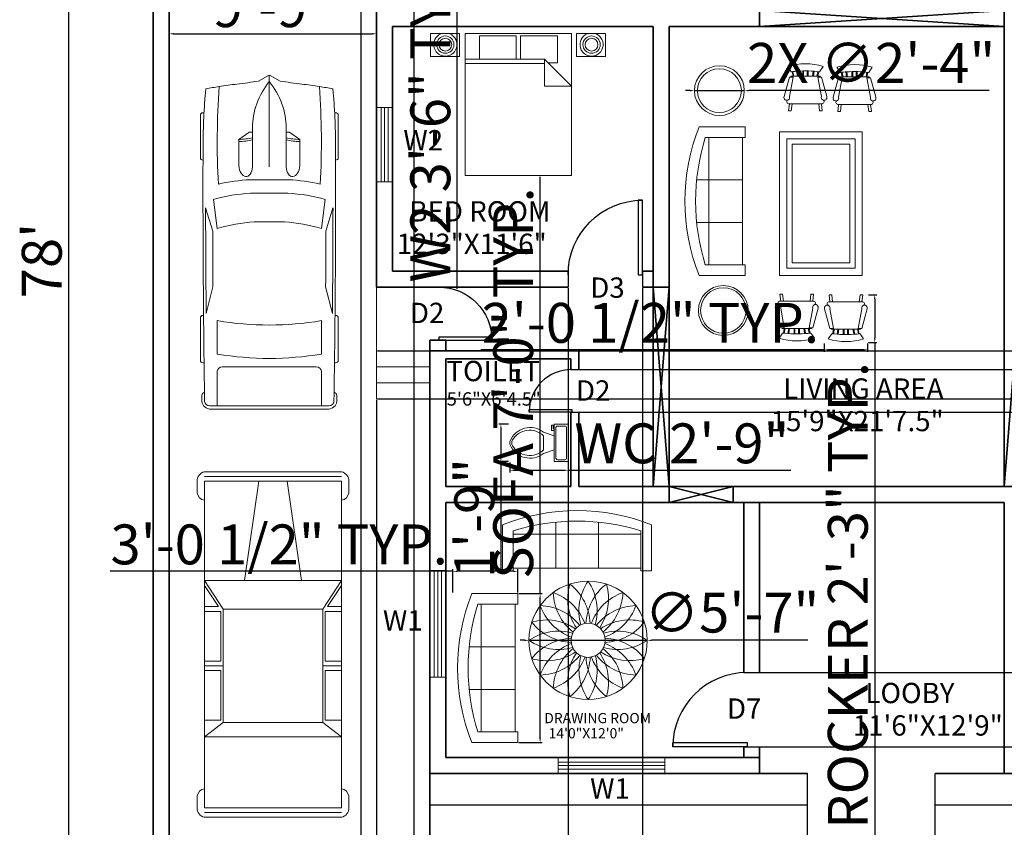
# Model space of a CAD drawing. Units: inches. Extents: x 164 to 1038, y 98 to 1358.
# Tile 2 of 4: x 199 to 754, y 358 to 814. Entities that reach past the tile are written whole.
import ezdxf

# ---------------------------------------------------------------- set-up
doc = ezdxf.new("R2010")
doc.units = ezdxf.units.IN
for name, color, linetype, lineweight in [('A-ANNO-DIMS', 7, 'Continuous', 18), ('A-ANNO-TEXT', 3, 'Continuous', 18), ('A-AREA-IDEN', 3, 'Continuous', 18), ('A-FLOR', 7, 'Continuous', 25), ('A-FLOR-FIXT', 2, 'Continuous', 18), ('C-SITE-VEHI', 2, 'Continuous', 13), ('C-SITE-WALL', 7, 'Continuous', 35), ('door', 6, 'Continuous', 25), ('furniture', 2, 'Continuous', 18), ('staircase', 4, 'Continuous', 18), ('wall', 7, 'Continuous', 35), ('window', 10, 'Continuous', 18)]:
    doc.layers.add(name, color=color, linetype=linetype, lineweight=lineweight)
doc.styles.get("Standard").update_dxf_attribs({"font": 'arial.ttf'})
doc.dimstyles.new('ISO-25', dxfattribs={"dimtxt": 22.5, "dimasz": 2.5, "dimexe": 1.25, "dimexo": 0.625, "dimtad": 1, "dimdec": 0, "dimlunit": 3, "dimtxsty": 'Standard', "dimcen": 2.5, "dimadec": 0, "dimazin": 0, "dimtfac": 1, "dimtdec": 0, "dimtmove": 0, "dimatfit": 3, "dimfxl": 1, "dimarcsym": 0})

# ---------------------------------------------------------------- blocks, each defined once
blk = doc.blocks.new('*U3')
for p, q in [((0, 0), (0, -5)), ((30, 0), (30, -5))]:
    blk.add_line(p, q)
blk.add_lwpolyline([(0, 0), (0, 30), (1.75, 30), (1.75, 0)], close=True)
blk.add_arc((0, 0), 30, 0, 90)
blk = doc.blocks.new('Bed - Queen')
for p, q in [((0, -80.00003), (0, 0)), ((0, 0), (59.99999, 0)), ((59.99999, 0), (59.99999, -80.00003)), ((7.99999, -1.2), (28.79998, -1.2)), ((7.99999, -14.4), (7.99999, -1.2)), ((28.79998, -1.2), (28.79998, -14.4)), ((31.19999, -1.2), (51.99999, -1.2)), ((31.19999, -14.4), (31.19999, -1.2)), ((51.99999, -1.2), (51.99999, -16.4)), ((0, -14.4), (44.8, -14.4)), ((59.99999, -29.6), (44.8, -14.4)), ((44.8, -14.4), (44.8, -29.6)), ((51.99999, -16.4), (46.79936, -16.4)), ((44.8, -16.8), (0, -16.8)), ((44.8, -29.6), (59.99999, -29.6)), ((59.99999, -80.00003), (0, -80.00003))]:
    blk.add_line(p, q)
blk = doc.blocks.new('Toilet - top')
for p, q in [((9.5, -6), (9.5, -2)), ((-10, -8.5), (-8, -8.5)), ((-10, -9.5), (-10, -8.5)), ((-7, -9.5), (-10, -9.5)), ((-8, -8.5), (-8, -8)), ((-7, -8), (-7, -9.5)), ((-4, -8), (-6, -14)), ((4, -8), (6, -14)), ((4, -14), (-4, -14))]:
    blk.add_line(p, q)
blk.add_lwpolyline([(10.5, -8), (10.5, 0), (-10.5, 0), (-10.5, -8)], close=True)
for points in [[(-9.5, -2), (-9.5, -6)], [(8.5, -1), (-8.5, -1)], [(-8.5, -7), (8.5, -7)]]:
    blk.add_lwpolyline(points)
for centre, radius, start, end in [((-8.62, -1.88), 0.884, 81.8699, 188.1301), ((8.62, -1.88), 0.884, 351.8699, 98.1301), ((-8.62, -6.12), 0.884, 171.8699, 278.1301), ((8.62, -6.12), 0.884, 261.8699, 8.1301), ((3.52, -21.58), 12.17, 141.4691, 247.9714), ((4.2, -21.82), 11.33, 136.3677, 238.9468), ((-3.52, -21.58), 12.17, 292.0284, 38.5307), ((-4.2, -21.82), 11.33, 301.053, 43.6321), ((0, -27.88), 4, 245.7318, 294.2682), ((0, -29), 4, 254.8605, 285.1395)]:
    blk.add_arc(centre, radius, start, end)
blk = doc.blocks.new('Sofa - Roundback 7 ft.')
for p, q in [((-12.00002, -32.4421), (-12.00003, -6.5971)), ((11.99997, -32.4421), (11.99998, -6.5971)), ((-36.000027, -34), (-36.000027, -11.4696)), ((-35.999844, -13.3819), (35.9998, -13.3819)), ((35.99998, -34), (35.99998, -11.4696)), ((-36.000027, -32.4421), (35.99998, -32.4421))]:
    blk.add_line(p, q)
for points in [[(-36.000027, -34), (-42.000027, -34), (-42.000027, -8)], [(41.99998, -8), (41.99998, -34), (35.99998, -34)]]:
    blk.add_lwpolyline(points)
for centre, radius, start, end in [((0, -114.25), 114.25, 68.43141, 111.5686), ((-0.00001, -127.1968), 121.1968, 72.72033, 107.2797)]:
    blk.add_arc(centre, radius, start, end)
blk = doc.blocks.new('Chair - Rocking')
for p, q in [((-8, -4.5), (-10, -1.5)), ((-7.5, -4.5), (-7, -7)), ((-6.5, -7), (-7.02225, -4.43)), ((-4.5, -7), (-4.96674, -4.19951)), ((-4, -7), (-4.40532, -4.16272)), ((-1.5, -4.05012), (-1.5, -7)), ((-1, -7), (-1, -4.05012)), ((1, -7), (1, -4.04655)), ((1.5, -4.05012), (1.5, -7)), ((4, -7), (4.40187, -4.18694)), ((4.5, -7), (4.96761, -4.19437)), ((6.5, -7), (7, -4.4057)), ((7.5, -4.5), (7, -7)), ((8, -4.5), (10, -1.5)), ((-9, -7.5), (-12, -18.49999)), ((-7, -7.5), (-9, -7.5)), ((-9, -18.49999), (-7, -7.5)), ((-8.23428, -6.99939), (-8.3093, -7.47958)), ((-8.23041, -7), (8.23915, -7)), ((7, -7.5), (9, -7.5)), ((9, -18.49999), (7, -7.5)), ((8.31071, -7.48854), (8.23449, -7.00073)), ((9, -7.5), (12, -18.49999)), ((-10.36644, -20.64523), (-10.5, -21.49999)), ((10.5, -21.49999), (10.3575, -20.58798)), ((-9, -22.49999), (-9.5, -26.49999)), ((0, -22.49999), (-9.5, -22.49999)), ((-9.5, -26.49999), (-8, -26.49999)), ((-8, -26.49999), (-7.5, -22.49999)), ((0, -22.49999), (9.5, -22.49999)), ((8, -26.49999), (7.5, -22.49999)), ((9.5, -26.49999), (8, -26.49999)), ((9, -22.49999), (9.5, -26.49999))]:
    blk.add_line(p, q)
for centre, radius, start, end in [((0, -34.08333), 34.08333, 72.93847, 107.0615), ((0, -68.25004), 64.25, 93.92211, 97.15267), ((0, -68.25004), 64.25, 82.84733, 93.92211), ((-10.5, -18.99999), 1.58114, 161.5651, 18.43495), ((-9.5, -21.49999), 1, 180, 270), ((10.5, -18.99999), 1.58114, 161.5651, 18.43495), ((9.5, -21.49999), 1, 270, 0)]:
    blk.add_arc(centre, radius, start, end)
blk = doc.blocks.new('*U6')
for p, q in [((46.55, 38.89), (22.35, 38.89)), ((136.7, 38.89), (160.9, 38.89)), ((21.1, 37.41), (21.1, 36.83)), ((47.8, 37.39), (47.8, 37.41)), ((87.99, 31.87), (74.76, 35.92)), ((134.31, 35.6), (119.29, 31.78)), ((135.45, 37.07), (135.45, 37.41)), ((162.15, 37.41), (162.15, 36.77)), ((186.47, -33.5), (186.47, 33.5)), ((70.03, 31.54), (86.41, 29.35)), ((138.42, 29.35), (157.25, 29.35)), ((186.47, 29.35), (167.01, 29.35)), ((188.4, -32.76), (188.4, 32.76)), ((164.52, 26.39), (164.52, -26.39)), ((32.27, 11.63), (36.13, 17.17)), ((36.13, 17.17), (50.94, 17.17)), ((32.12, 9.51), (32.12, 11.15)), ((3.27, 6.13), (0.1, 0.41)), ((29.77, 9.51), (51.68, 9.51)), ((58.92, -10.77), (58.92, 10.77)), ((66.55, -10.53), (66.55, 10.53)), ((82.74, 8.5), (82.74, -8.5)), ((186.47, -10.53), (186.47, 10.53)), ((0, 0), (51.68, 0)), ((0.1, -0.41), (3.27, -6.13)), ((29.77, -9.51), (51.68, -9.51)), ((32.12, -9.51), (32.12, -11.15)), ((32.27, -11.63), (36.13, -17.17)), ((36.13, -17.17), (50.94, -17.17)), ((86.41, -29.35), (70.03, -31.54)), ((87.99, -31.87), (74.76, -35.92)), ((134.31, -35.6), (119.29, -31.78)), ((157.25, -29.35), (138.42, -29.35)), ((167.01, -29.35), (186.47, -29.35)), ((21.1, -37.41), (21.1, -36.83)), ((47.8, -37.39), (47.8, -37.41)), ((135.45, -37.07), (135.45, -37.41)), ((162.15, -37.41), (162.15, -36.77)), ((46.55, -38.89), (22.35, -38.89)), ((136.7, -38.89), (160.9, -38.89))]:
    blk.add_line(p, q)
for centre, major_axis, ratio, start_param, end_param in [((22.35, 37.41), (0, -1.48), 0.842304, 3.141593, 4.712389), ((46.55, 37.41), (0, 1.48), 0.842304, -1.570796, 0), ((136.7, 37.41), (0, -1.48), 0.842304, 3.141593, 4.712389), ((160.9, 37.41), (0, 1.48), 0.842304, -1.570796, 0), ((266.03, -27.52), (0, 313.31), 0.842304, 1.367076, 1.39176), ((41.19, -490.86), (0, 528.23), 0.842304, 0.00281, 0.075598), ((64.48, -10555.62), (0, 10593.03), 0.842304, -0.013397, 0.002797), ((64.48, -10555.62), (0, -10591.55), 0.842304, 3.133765, 3.140441), ((180.63, 35.84), (0, 2.22), 0.842304, -0.013017, 1.249894), ((64.48, -10556.36), (0, 10595.31), 0.842304, -0.013397, -0.013017), ((183.98, 33.5), (0, -2.96), 0.842304, 1.570796, 3.128196), ((183.98, 32.76), (0, -5.25), 0.842304, 1.570796, 3.128196), ((259.18, -27.52), (0, -305.3), 0.842304, 4.528606, 4.561838), ((37.47, -593.96), (0, -623.33), 0.842304, 3.096046, 3.200911), ((134.4, 5.39), (0, -89.78), 0.842304, 4.449482, 4.652344), ((135.29, 5.39), (0, 81.77), 0.842304, 1.245306, 1.50788), ((149.6, 2.8), (0, -79.58), 0.842304, 4.372215, 4.640744), ((95.79, -3666.35), (0, -3698.24), 0.842304, 3.134049, 3.144098), ((17.08, 0), (0, 147.02), 0.842304, 4.511394, 4.913384), ((35.91, 0), (0, 147.02), 0.842304, 4.511394, 4.913384), ((167.01, 26.39), (0, 2.96), 0.842304, 0, 1.570796), ((-204.49, 52.4), (0, -250.96), 0.842304, 1.385369, 1.434372), ((13.04, 17.01), (0, 27.42), 0.842304, 4.435146, 4.718221), ((14.2, 17.01), (0, 27.42), 0.842304, 4.435146, 4.718221), ((50.79, 13.34), (6.34, -0.36), 0.603834, -1.395552, 1.581315), ((32.75, 11.15), (0, 0.74), 0.842304, 0.879714, 1.570796), ((29.77, -46.66), (0, 56.17), 0.842304, 0, 0.590319), ((0.62, 0), (0, -0.74), 0.842304, 4.131459, 5.293319), ((29.77, 46.66), (0, 56.17), 0.842304, 2.551274, 3.141593), ((-204.49, -52.4), (0, 250.96), 0.842304, -1.434372, -1.385369), ((13.04, -17.01), (0, -27.42), 0.842304, 1.564964, 1.848039), ((14.2, -17.01), (0, -27.42), 0.842304, 1.564964, 1.848039), ((134.4, -5.39), (0, -89.78), 0.842304, -1.510751, -1.307889), ((135.29, -5.39), (0, -81.77), 0.842304, -1.50788, -1.245306), ((149.6, -2.8), (0, -79.58), 0.842304, -1.499151, -1.230623), ((32.75, -11.15), (0, -0.74), 0.842304, 4.712389, 5.403472), ((259.18, 27.52), (0, 305.3), 0.842304, 1.721348, 1.754579), ((167.01, -26.39), (0, -2.96), 0.842304, 4.712389, 6.283185), ((266.03, 27.52), (0, 313.31), 0.842304, 1.749832, 1.774517), ((37.47, 593.96), (0, -623.33), 0.842304, -0.059319, 0.045547), ((95.79, 3666.35), (0, -3698.24), 0.842304, -0.002505, 0.007544), ((183.98, -32.76), (0, -5.25), 0.842304, 0.013397, 1.570796), ((41.19, 490.86), (0, -528.23), 0.842304, -0.075598, -0.00281), ((22.35, -37.41), (0, 1.48), 0.842304, 1.570796, 3.141593), ((64.48, 10555.62), (0, 10593.03), 0.842304, 3.138796, 3.15499), ((46.55, -37.41), (0, -1.48), 0.842304, 0, 1.570796), ((64.48, 10555.62), (0, -10591.55), 0.842304, 0.001152, 0.007828), ((136.7, -37.41), (0, -1.48), 0.842304, -1.570796, 0), ((160.9, -37.41), (0, 1.48), 0.842304, 3.141593, 4.712389), ((180.63, -35.84), (0, -2.22), 0.842304, -1.249894, 0.013017), ((64.48, 10556.36), (0, 10595.31), 0.842304, 3.15461, 3.15499), ((183.98, -33.5), (0, 2.96), 0.842304, 3.15499, 4.712389)]:
    blk.add_ellipse(centre, major_axis=major_axis, ratio=ratio, start_param=start_param, end_param=end_param)
at = {"extrusion": (0, 0, -1)}
blk.add_ellipse((50.79, -13.34), major_axis=(6.34, 0.36), ratio=0.603834, start_param=-1.395552, end_param=1.581315, dxfattribs=at)
blk = doc.blocks.new('*U14')
for p, q in [((5.44, 42.31), (12.12, 42.31)), ((189.69, 42.31), (183.01, 42.31)), ((0.1, -0.41), (0.1, 38.35)), ((2.77, -0.41), (2.77, 38.31)), ((5.44, -0.41), (5.44, 38.24)), ((5.45, 38.31), (16.12, 38.31)), ((16.12, 38.31), (180.34, 38.31)), ((61.52, -0.41), (61.52, 38.31)), ((61.52, 38.31), (77.54, 27.62)), ((64.19, 38.31), (76.2, 30.29)), ((76.2, 30.29), (76.2, 38.31)), ((78.87, 38.31), (78.87, 28.96)), ((106.91, 28.96), (106.91, 38.31)), ((109.58, 27.62), (109.58, 38.31)), ((112.25, 38.31), (112.25, 28.96)), ((140.29, 28.96), (140.29, 38.31)), ((141.62, 27.62), (149.64, 38.31)), ((149.64, -0.41), (149.64, 38.31)), ((189.69, 38.31), (179.01, 38.31)), ((189.69, -0.41), (189.69, 38.24)), ((192.36, -0.41), (192.36, 38.31)), ((195.03, -0.41), (195.03, 38.35)), ((78.87, 28.96), (106.91, 28.96)), ((112.25, 28.96), (140.29, 28.96)), ((77.54, 27.62), (141.62, 27.62)), ((77.54, -0.41), (77.54, 27.62)), ((141.62, -0.41), (141.62, 27.62)), ((5.44, 7.6), (61.52, 15.61)), ((0.1, -0.42), (0.1, -39.18)), ((2.77, -0.41), (2.77, -39.13)), ((5.44, -0.42), (5.44, -39.07)), ((61.52, -0.41), (61.52, -39.13)), ((77.54, -0.41), (77.54, -28.45)), ((141.62, -0.41), (141.62, -28.45)), ((149.64, -0.41), (149.64, -39.13)), ((189.69, -0.42), (189.69, -39.07)), ((192.36, -0.41), (192.36, -39.13)), ((195.03, -0.42), (195.03, -39.18)), ((5.44, -8.42), (61.52, -16.43)), ((61.52, -39.13), (77.54, -28.45)), ((64.19, -39.13), (76.2, -31.12)), ((76.2, -31.12), (76.2, -39.13)), ((77.54, -28.45), (141.62, -28.45)), ((78.87, -39.13), (78.87, -29.79)), ((78.87, -29.79), (106.91, -29.79)), ((106.91, -29.79), (106.91, -39.13)), ((109.58, -28.45), (109.58, -39.13)), ((112.25, -29.79), (140.29, -29.79)), ((112.25, -39.13), (112.25, -29.79)), ((140.29, -29.79), (140.29, -39.13)), ((141.62, -28.45), (149.64, -39.13)), ((5.44, -43.14), (12.12, -43.14)), ((5.45, -39.13), (16.12, -39.13)), ((16.12, -39.13), (180.34, -39.13)), ((189.69, -39.13), (179.01, -39.13)), ((189.69, -43.14), (183.01, -43.14))]:
    blk.add_line(p, q)
for centre, radius, start, end in [((5.06, 37.26), 5.06, 85.6455, 168.0943), ((11.45, 37.64), 4.72, 8.1301, 81.87), ((183.68, 37.64), 4.72, 98.13, 171.8699), ((190.07, 37.26), 5.06, 11.9057, 94.3545), ((5.06, -38.09), 5.06, 191.9057, 274.3545), ((11.45, -38.46), 4.72, 278.13, 351.8699), ((183.68, -38.46), 4.72, 188.1301, 261.87), ((190.07, -38.09), 5.06, 265.6455, 348.0943)]:
    blk.add_arc(centre, radius, start, end)
blk = doc.blocks.new('*U15')
at = {"layer": 'furniture'}
for centre, radius, start, end in [((24.35, -4.35), 29.51, 145.5556, 195.7248), ((-24.51, -4.35), 29.67, 344.3816, 34.2394)]:
    blk.add_arc(centre, radius, start, end, dxfattribs=at)
blk = doc.blocks.new('*U16')
at = {"layer": 'furniture', "transparency": 16777216}
for p, rotation in [((298.67, 483.56), 18.00000000000003), ((311.67, 483.57), 342.0000000000001), ((292.8, 480.57), 36.00000000000004), ((317.54, 480.59), 324.0000000000001), ((288.15, 475.91), 54.00000000000005), ((322.2, 475.94), 306), ((285.17, 470.04), 72.00000000000006), ((325.19, 470.07), 288.0000000000001), ((284.14, 463.54), 90.00000000000006), ((326.22, 463.57), 270.0000000000001), ((285.18, 457.04), 108), ((288.17, 451.18), 126), ((322.21, 451.2), 234), ((325.2, 457.07), 252), ((292.83, 446.52), 144), ((298.7, 443.54), 162), ((311.7, 443.55), 198), ((317.56, 446.54), 216), ((305.2, 442.52), 180)]:
    blk.add_blockref('*U15', p, dxfattribs=dict(at, rotation=rotation))
blk.add_blockref('*U15', (305.17, 484.59), dxfattribs=at)
blk = doc.blocks.new('*D20')
at = {"layer": 'A-ANNO-DIMS', "color": 0, "lineweight": -2, "transparency": 16777216}
for p, q in [((273.44, 1145.87), (224.94, 1145.87)), ((226.19, 1143.37), (226.19, 212.37)), ((273.44, 209.87), (224.94, 209.87))]:
    blk.add_line(p, q, dxfattribs=at)
at = {"layer": 'A-ANNO-DIMS', "color": 0, "transparency": 16777216}
for points in [[(225.78, 1143.37), (226.61, 1143.37), (226.19, 1145.87)], [(225.78, 212.37), (226.61, 212.37), (226.19, 209.87)]]:
    blk.add_solid(points, dxfattribs=at)
at = {"layer": 'Defpoints', "color": 0, "transparency": 16777216}
for p in [(274.07, 1145.87), (226.19, 209.87), (274.07, 209.87)]:
    blk.add_point(p, dxfattribs=at)
at = {"layer": 'A-ANNO-DIMS', "color": 0, "transparency": 16777216, "insert": (214.08, 677.87), "char_height": 22.5, "attachment_point": 5, "rotation": 90}
blk.add_mtext("78'", dxfattribs=at)
blk = doc.blocks.new('*D24')
at = {"layer": 'A-ANNO-DIMS', "color": 0, "lineweight": -2, "transparency": 16777216}
for p, q in [((283.07, 795.15), (283.07, 807.04)), ((285.57, 805.79), (397.57, 805.79)), ((400.07, 795.15), (400.07, 807.04))]:
    blk.add_line(p, q, dxfattribs=at)
at = {"layer": 'A-ANNO-DIMS', "color": 0, "transparency": 16777216}
for points in [[(285.57, 806.21), (285.57, 805.37), (283.07, 805.79)], [(397.57, 806.21), (397.57, 805.37), (400.07, 805.79)]]:
    blk.add_solid(points, dxfattribs=at)
at = {"layer": 'Defpoints', "color": 0, "transparency": 16777216}
for p in [(400.07, 805.79), (283.07, 794.52), (400.07, 794.52)]:
    blk.add_point(p, dxfattribs=at)
at = {"layer": 'A-ANNO-DIMS', "color": 0, "transparency": 16777216, "insert": (341.57, 817.9), "char_height": 22.5, "attachment_point": 5}
blk.add_mtext('9\'-9"', dxfattribs=at)
blk = doc.blocks.new('WINDOW-W1')
for p, q in [((0, 9), (0, 0)), ((0, 6.5), (60.11, 6.5)), ((60.11, 9), (60.11, 0)), ((0, 4.5), (60.11, 4.5)), ((0, 2.5), (60.11, 2.5))]:
    blk.add_line(p, q)
blk = doc.blocks.new('WINDOW-W2')
for p, q in [((0, 9), (0, 0)), ((0, 6.5), (42.02, 6.5)), ((42.02, 9), (42.02, 0)), ((0, 4.5), (42.02, 4.5)), ((0, 2.5), (42.02, 2.5))]:
    blk.add_line(p, q)
blk = doc.blocks.new('BEDSIDE-TABLE')
blk.add_lwpolyline([(0, 13.01), (16.36, 13.01), (16.36, 0), (0, 0)], close=True)
for radius in [4.87, 3.63]:
    blk.add_circle((8.46, 6.65), radius)
blk.add_arc((8.46, 6.65), 6.51, 102.0293, 77.9707)
blk.add_arc((8.46, 6.65), 6.51, 102.0293, 77.9707)
blk = doc.blocks.new('*D36')
at = {"layer": 'A-ANNO-DIMS', "color": 0, "lineweight": -2, "transparency": 16777216}
for p, q in [((439.69, 901.66), (446.62, 901.66)), ((445.37, 899.16), (445.37, 862.14)), ((439.69, 859.64), (446.62, 859.64)), ((445.37, 859.64), (445.37, 661.94))]:
    blk.add_line(p, q, dxfattribs=at)
at = {"layer": 'A-ANNO-DIMS', "color": 0, "transparency": 16777216}
for points in [[(444.95, 899.16), (445.79, 899.16), (445.37, 901.66)], [(444.95, 862.14), (445.79, 862.14), (445.37, 859.64)]]:
    blk.add_solid(points, dxfattribs=at)
at = {"layer": 'Defpoints', "color": 0, "transparency": 16777216}
for p in [(439.07, 901.66), (439.07, 859.64), (445.37, 859.64)]:
    blk.add_point(p, dxfattribs=at)
at = {"layer": 'A-ANNO-DIMS', "color": 0, "transparency": 16777216, "insert": (433.25, 759.54), "char_height": 22.5, "attachment_point": 5, "rotation": 90}
blk.add_mtext('W2 3\'-6" TYP.', dxfattribs=at)
blk = doc.blocks.new('*D44')
at = {"layer": 'A-ANNO-DIMS', "color": 0, "lineweight": -2, "transparency": 16777216}
for p, q in [((677.56, 658.58), (682.23, 658.58)), ((680.98, 656.08), (680.98, 634.08)), ((677.56, 631.58), (682.23, 631.58)), ((680.98, 631.58), (680.98, 348.63))]:
    blk.add_line(p, q, dxfattribs=at)
at = {"layer": 'A-ANNO-DIMS', "color": 0, "transparency": 16777216}
for points in [[(680.57, 656.08), (681.4, 656.08), (680.98, 658.58)], [(680.57, 634.08), (681.4, 634.08), (680.98, 631.58)]]:
    blk.add_solid(points, dxfattribs=at)
at = {"layer": 'Defpoints', "color": 0, "transparency": 16777216}
for p in [(676.93, 658.58), (676.93, 631.58), (680.98, 631.58)]:
    blk.add_point(p, dxfattribs=at)
at = {"layer": 'A-ANNO-DIMS', "color": 0, "transparency": 16777216, "insert": (668.71, 488.85), "char_height": 22.5, "attachment_point": 5, "rotation": 90}
blk.add_mtext('ROCKER 2\'-3" TYP.', dxfattribs=at)
blk = doc.blocks.new('*D45')
at = {"layer": 'A-ANNO-DIMS', "color": 0, "lineweight": -2, "transparency": 16777216}
for p, q in [((652.5, 627.53), (458.79, 627.53)), ((652.5, 630.95), (652.5, 626.28)), ((674.43, 627.53), (655, 627.53)), ((676.93, 630.95), (676.93, 626.28))]:
    blk.add_line(p, q, dxfattribs=at)
at = {"layer": 'A-ANNO-DIMS', "color": 0, "transparency": 16777216}
for points in [[(655, 627.94), (655, 627.11), (652.5, 627.53)], [(674.43, 627.94), (674.43, 627.11), (676.93, 627.53)]]:
    blk.add_solid(points, dxfattribs=at)
at = {"layer": 'Defpoints', "color": 0, "transparency": 16777216}
for p in [(652.5, 631.58), (652.5, 627.53), (676.93, 631.58)]:
    blk.add_point(p, dxfattribs=at)
at = {"layer": 'A-ANNO-DIMS', "color": 0, "transparency": 16777216, "insert": (554.39, 639.78), "char_height": 22.5, "attachment_point": 5}
blk.add_mtext('2\'-0 1/2" TYP.', dxfattribs=at)
blk = doc.blocks.new('*D46')
at = {"layer": 'A-ANNO-DIMS', "color": 0, "lineweight": -2, "transparency": 16777216}
for p, q in [((492.26, 489.89), (492.26, 725)), ((480.29, 489.89), (493.51, 489.89)), ((492.26, 408.39), (492.26, 487.39)), ((480.29, 405.89), (493.51, 405.89))]:
    blk.add_line(p, q, dxfattribs=at)
at = {"layer": 'A-ANNO-DIMS', "color": 0, "transparency": 16777216}
for points in [[(491.84, 487.39), (492.68, 487.39), (492.26, 489.89)], [(491.84, 408.39), (492.68, 408.39), (492.26, 405.89)]]:
    blk.add_solid(points, dxfattribs=at)
at = {"layer": 'Defpoints', "color": 0, "transparency": 16777216}
for p in [(479.66, 489.89), (492.26, 489.89), (479.66, 405.89)]:
    blk.add_point(p, dxfattribs=at)
at = {"layer": 'A-ANNO-DIMS', "color": 0, "transparency": 16777216, "insert": (479.99, 608.7), "char_height": 22.5, "attachment_point": 5, "rotation": 90}
blk.add_mtext('SOFA 7\'-0" TYP.', dxfattribs=at)
blk = doc.blocks.new('*D47')
at = {"layer": 'A-ANNO-DIMS', "color": 0, "lineweight": -2, "transparency": 16777216}
for p, q in [((442.99, 502.49), (249.68, 502.49)), ((442.99, 490.52), (442.99, 503.74)), ((477.16, 502.49), (445.49, 502.49)), ((479.66, 490.52), (479.66, 503.74))]:
    blk.add_line(p, q, dxfattribs=at)
at = {"layer": 'A-ANNO-DIMS', "color": 0, "transparency": 16777216}
for points in [[(445.49, 502.91), (445.49, 502.08), (442.99, 502.49)], [(477.16, 502.91), (477.16, 502.08), (479.66, 502.49)]]:
    blk.add_solid(points, dxfattribs=at)
at = {"layer": 'Defpoints', "color": 0, "transparency": 16777216}
for p in [(442.99, 502.49), (442.99, 489.89), (479.66, 489.89)]:
    blk.add_point(p, dxfattribs=at)
at = {"layer": 'A-ANNO-DIMS', "color": 0, "transparency": 16777216, "insert": (345.09, 514.76), "char_height": 22.5, "attachment_point": 5}
blk.add_mtext('3\'-0 1/2" TYP.', dxfattribs=at)
blk = doc.blocks.new('*D50')
at = {"layer": 'A-ANNO-DIMS', "color": 0, "lineweight": -2, "transparency": 16777216}
for p, q in [((475.12, 563.85), (475.12, 558.27)), ((508.17, 563.85), (508.17, 558.27)), ((477.62, 559.52), (505.67, 559.52)), ((508.17, 559.52), (633.75, 559.52))]:
    blk.add_line(p, q, dxfattribs=at)
at = {"layer": 'A-ANNO-DIMS', "color": 0, "transparency": 16777216}
for points in [[(477.62, 559.94), (477.62, 559.1), (475.12, 559.52)], [(505.67, 559.94), (505.67, 559.1), (508.17, 559.52)]]:
    blk.add_solid(points, dxfattribs=at)
at = {"layer": 'Defpoints', "color": 0, "transparency": 16777216}
for p in [(475.12, 564.48), (508.17, 564.48), (508.17, 559.52)]:
    blk.add_point(p, dxfattribs=at)
at = {"layer": 'A-ANNO-DIMS', "color": 0, "transparency": 16777216, "insert": (572.21, 571.78), "char_height": 22.5, "attachment_point": 5}
blk.add_mtext('WC 2\'-9"', dxfattribs=at)
blk = doc.blocks.new('*D51')
at = {"layer": 'A-ANNO-DIMS', "color": 0, "lineweight": -2, "transparency": 16777216}
for p, q in [((474.5, 585.48), (468.91, 585.48)), ((470.16, 582.98), (470.16, 566.98)), ((474.5, 564.48), (468.91, 564.48)), ((470.16, 564.48), (470.16, 503.03))]:
    blk.add_line(p, q, dxfattribs=at)
at = {"layer": 'A-ANNO-DIMS', "color": 0, "transparency": 16777216}
for points in [[(469.75, 582.98), (470.58, 582.98), (470.16, 585.48)], [(469.75, 566.98), (470.58, 566.98), (470.16, 564.48)]]:
    blk.add_solid(points, dxfattribs=at)
at = {"layer": 'Defpoints', "color": 0, "transparency": 16777216}
for p in [(475.12, 585.48), (470.16, 564.48), (475.12, 564.48)]:
    blk.add_point(p, dxfattribs=at)
at = {"layer": 'A-ANNO-DIMS', "color": 0, "transparency": 16777216, "insert": (458.05, 532.51), "char_height": 22.5, "attachment_point": 5, "rotation": 90}
blk.add_mtext('1\'-9"', dxfattribs=at)
blk = doc.blocks.new('*D54')
at = {"layer": 'A-ANNO-DIMS', "color": 0, "lineweight": -2, "transparency": 16777216}
for p, q in [((391.07, 1028.24), (391.07, 152.07)), ((421.07, 1028.24), (421.07, 152.07)), ((393.57, 153.32), (418.57, 153.32)), ((421.07, 153.32), (485.01, 153.32))]:
    blk.add_line(p, q, dxfattribs=at)
at = {"layer": 'A-ANNO-DIMS', "color": 0, "transparency": 16777216}
for points in [[(393.57, 153.73), (393.57, 152.9), (391.07, 153.32)], [(418.57, 153.73), (418.57, 152.9), (421.07, 153.32)]]:
    blk.add_solid(points, dxfattribs=at)
at = {"layer": 'Defpoints', "color": 0, "transparency": 16777216}
for p in [(391.07, 1028.87), (421.07, 1028.87), (421.07, 153.32)]:
    blk.add_point(p, dxfattribs=at)
at = {"layer": 'A-ANNO-DIMS', "color": 0, "transparency": 16777216, "insert": (454.29, 165.43), "char_height": 22.5, "attachment_point": 5}
blk.add_mtext('2\'-6"', dxfattribs=at)
blk = doc.blocks.new('*D55')
at = {"layer": 'A-ANNO-DIMS', "color": 0, "lineweight": -2, "transparency": 16777216}
for p, q in [((508.07, 662.24), (508.07, 152.07)), ((550.07, 662.24), (550.07, 152.07)), ((510.57, 153.32), (547.57, 153.32)), ((550.07, 153.32), (613.61, 153.32))]:
    blk.add_line(p, q, dxfattribs=at)
at = {"layer": 'A-ANNO-DIMS', "color": 0, "transparency": 16777216}
for points in [[(510.57, 153.73), (510.57, 152.9), (508.07, 153.32)], [(547.57, 153.73), (547.57, 152.9), (550.07, 153.32)]]:
    blk.add_solid(points, dxfattribs=at)
at = {"layer": 'Defpoints', "color": 0, "transparency": 16777216}
for p in [(508.07, 662.87), (550.07, 662.87), (550.07, 153.32)]:
    blk.add_point(p, dxfattribs=at)
at = {"layer": 'A-ANNO-DIMS', "color": 0, "transparency": 16777216, "insert": (583.09, 165.44), "char_height": 22.5, "attachment_point": 5}
blk.add_mtext('3\'-6"', dxfattribs=at)
blk = doc.blocks.new('*D56')
at = {"layer": 'A-ANNO-DIMS', "color": 0, "lineweight": -2, "transparency": 16777216}
for p, q in [((1035.62, 616.37), (1035.62, 680.31)), ((510.19, 616.37), (1036.87, 616.37)), ((1035.62, 594.87), (1035.62, 613.87)), ((510.19, 592.37), (1036.87, 592.37))]:
    blk.add_line(p, q, dxfattribs=at)
at = {"layer": 'A-ANNO-DIMS', "color": 0, "transparency": 16777216}
for points in [[(1035.2, 613.87), (1036.03, 613.87), (1035.62, 616.37)], [(1035.2, 594.87), (1036.03, 594.87), (1035.62, 592.37)]]:
    blk.add_solid(points, dxfattribs=at)
at = {"layer": 'Defpoints', "color": 0, "transparency": 16777216}
for p in [(509.57, 616.37), (1035.62, 616.37), (509.57, 592.37)]:
    blk.add_point(p, dxfattribs=at)
at = {"layer": 'A-ANNO-DIMS', "color": 0, "transparency": 16777216, "insert": (1023.5, 649.59), "char_height": 22.5, "attachment_point": 5, "rotation": 90}
blk.add_mtext('2\'-0"', dxfattribs=at)
blk = doc.blocks.new('*D57')
at = {"layer": 'A-ANNO-DIMS', "color": 0, "lineweight": -2, "transparency": 16777216}
for p, q in [((400.07, 599.24), (400.07, 152.07)), ((430.07, 599.24), (430.07, 152.07)), ((402.57, 153.32), (427.57, 153.32)), ((430.07, 153.32), (494.01, 153.32))]:
    blk.add_line(p, q, dxfattribs=at)
at = {"layer": 'A-ANNO-DIMS', "color": 0, "transparency": 16777216}
for points in [[(402.57, 153.73), (402.57, 152.9), (400.07, 153.32)], [(427.57, 153.73), (427.57, 152.9), (430.07, 153.32)]]:
    blk.add_solid(points, dxfattribs=at)
at = {"layer": 'Defpoints', "color": 0, "transparency": 16777216}
for p in [(400.07, 599.87), (430.07, 599.87), (430.07, 153.32)]:
    blk.add_point(p, dxfattribs=at)
at = {"layer": 'A-ANNO-DIMS', "color": 0, "transparency": 16777216, "insert": (463.29, 165.43), "char_height": 22.5, "attachment_point": 5}
blk.add_mtext('2\'-6"', dxfattribs=at)
blk = doc.blocks.new('*D58')
at = {"layer": 'A-ANNO-DIMS', "color": 0, "lineweight": -2, "transparency": 16777216}
for p, q in [((1035.62, 626.87), (1035.62, 690.81)), ((400.69, 626.87), (1036.87, 626.87)), ((1035.62, 602.37), (1035.62, 624.37)), ((400.69, 599.87), (1036.87, 599.87))]:
    blk.add_line(p, q, dxfattribs=at)
at = {"layer": 'A-ANNO-DIMS', "color": 0, "transparency": 16777216}
for points in [[(1035.2, 624.37), (1036.03, 624.37), (1035.62, 626.87)], [(1035.2, 602.37), (1036.03, 602.37), (1035.62, 599.87)]]:
    blk.add_solid(points, dxfattribs=at)
at = {"layer": 'Defpoints', "color": 0, "transparency": 16777216}
for p in [(400.07, 626.87), (1035.62, 626.87), (400.07, 599.87)]:
    blk.add_point(p, dxfattribs=at)
at = {"layer": 'A-ANNO-DIMS', "color": 0, "transparency": 16777216, "insert": (1023.5, 660.09), "char_height": 22.5, "attachment_point": 5, "rotation": 90}
blk.add_mtext('2\'-3"', dxfattribs=at)
blk = doc.blocks.new('*D59')
at = {"layer": 'A-ANNO-DIMS', "color": 0, "lineweight": -2, "transparency": 16777216}
for p, q in [((1035.62, 445.37), (1035.62, 508.91)), ((607.69, 445.37), (1036.87, 445.37)), ((1035.62, 405.87), (1035.62, 442.87)), ((607.69, 403.37), (1036.87, 403.37))]:
    blk.add_line(p, q, dxfattribs=at)
at = {"layer": 'A-ANNO-DIMS', "color": 0, "transparency": 16777216}
for points in [[(1035.2, 442.87), (1036.03, 442.87), (1035.62, 445.37)], [(1035.2, 405.87), (1036.03, 405.87), (1035.62, 403.37)]]:
    blk.add_solid(points, dxfattribs=at)
at = {"layer": 'Defpoints', "color": 0, "transparency": 16777216}
for p in [(607.07, 445.37), (1035.62, 445.37), (607.07, 403.37)]:
    blk.add_point(p, dxfattribs=at)
at = {"layer": 'A-ANNO-DIMS', "color": 0, "transparency": 16777216, "insert": (1023.5, 478.39), "char_height": 22.5, "attachment_point": 5, "rotation": 90}
blk.add_mtext('3\'-6"', dxfattribs=at)
blk = doc.blocks.new('*D62')
at = {"layer": 'A-ANNO-DIMS', "color": 0, "lineweight": -2, "transparency": 16777216}
for p, q in [((483.44, 463.56), (480.94, 463.56)), ((485.94, 463.56), (552.71, 463.56)), ((643.25, 463.56), (555.21, 463.56))]:
    blk.add_line(p, q, dxfattribs=at)
at = {"layer": 'A-ANNO-DIMS', "color": 0, "transparency": 16777216}
for points in [[(483.44, 463.97), (483.44, 463.14), (485.94, 463.56)], [(555.21, 463.97), (555.21, 463.14), (552.71, 463.56)]]:
    blk.add_solid(points, dxfattribs=at)
at = {"layer": 'Defpoints', "color": 0, "transparency": 16777216}
for p in [(485.94, 463.56), (552.71, 463.56)]:
    blk.add_point(p, dxfattribs=at)
at = {"layer": 'A-ANNO-DIMS', "color": 0, "transparency": 16777216, "insert": (600.48, 476.3), "char_height": 22.5, "attachment_point": 5, "rotation": 0.0008}
blk.add_mtext('∅5\'-7"', dxfattribs=at)
blk = doc.blocks.new('*D63')
at = {"layer": 'A-ANNO-DIMS', "color": 0, "lineweight": -2, "transparency": 16777216}
for p, q in [((576.82, 773.71), (574.32, 773.71)), ((579.32, 773.71), (607.44, 773.71)), ((745.52, 773.71), (609.94, 773.71))]:
    blk.add_line(p, q, dxfattribs=at)
at = {"layer": 'A-ANNO-DIMS', "color": 0, "transparency": 16777216}
for points in [[(576.82, 774.13), (576.82, 773.29), (579.32, 773.71)], [(609.94, 774.13), (609.94, 773.29), (607.44, 773.71)]]:
    blk.add_solid(points, dxfattribs=at)
at = {"layer": 'Defpoints', "color": 0, "transparency": 16777216}
for p in [(579.32, 773.71), (607.44, 773.71)]:
    blk.add_point(p, dxfattribs=at)
at = {"layer": 'A-ANNO-DIMS', "color": 0, "transparency": 16777216, "insert": (678.98, 786.45), "char_height": 22.5, "attachment_point": 5, "rotation": 360}
blk.add_mtext('2X ∅2\'-4"', dxfattribs=at)

msp = doc.modelspace()

# ---------------------------------------------------------------- linework, layer by layer
at = {"layer": 'A-FLOR'}
for p, q in [((643.07, 352.37), (643.07, 388.37)), ((715.07, 352.37), (715.07, 388.37)), ((430.07, 370.73), (643.07, 370.73)), ((715.07, 370.73), (928.07, 370.73))]:
    msp.add_line(p, q, dxfattribs=at)
at = {"layer": 'C-SITE-WALL'}
for p, q in [((274.07, 1145.87), (274.07, 209.87)), ((283.07, 1028.87), (283.07, 662.87)), ((283.07, 662.87), (283.07, 218.87))]:
    msp.add_line(p, q, dxfattribs=at)
at = {"layer": 'door'}
for p, q in [((508.07, 671.87), (508.07, 662.87)), ((550.07, 671.87), (550.07, 662.87)), ((509.57, 616.37), (514.07, 616.37)), ((509.57, 592.37), (514.07, 592.37)), ((607.07, 445.37), (616.07, 445.37)), ((607.07, 403.37), (616.07, 403.37))]:
    msp.add_line(p, q, dxfattribs=at)
at = {"layer": 'furniture'}
for points in [[(627.35, 750.45), (673.93, 750.45), (673.93, 669.47), (627.35, 669.47)], [(631.35, 746.45), (669.93, 746.45), (669.93, 673.47), (631.35, 673.47)], [(634.35, 743.45), (666.93, 743.45), (666.93, 676.47), (634.35, 676.47)]]:
    msp.add_lwpolyline(points, close=True, dxfattribs=at)
for centre, radius in [((593.38, 773.71), 14.06), ((593.38, 773.71), 14.06), ((593.38, 773.71), 12.39), ((595.59, 649.68), 14.06), ((595.59, 649.68), 12.83), ((519.32, 463.56), 33.38), ((519.32, 463.56), 9.6)]:
    msp.add_circle(centre, radius, dxfattribs=at)
at = {"layer": 'staircase'}
for p, q in [((400.07, 662.87), (400.07, 599.87)), ((430.07, 626.87), (400.07, 626.87)), ((430.07, 617.87), (400.07, 617.87)), ((430.07, 608.87), (400.07, 608.87)), ((430.07, 599.87), (400.07, 599.87))]:
    msp.add_line(p, q, dxfattribs=at)
at = {"layer": 'wall'}
for p, q in [((616.07, 824.87), (616.07, 809.87)), ((400.07, 818.87), (400.07, 662.87)), ((616.07, 818.87), (754.07, 809.87)), ((754.07, 818.87), (616.07, 809.87)), ((754.07, 818.87), (754.07, 550.37)), ((409.07, 809.87), (409.07, 671.87)), ((556.07, 809.87), (409.07, 809.87)), ((556.07, 809.87), (556.07, 550.37)), ((565.07, 809.87), (565.07, 550.37)), ((754.07, 809.87), (565.07, 809.87)), ((508.07, 671.87), (409.07, 671.87)), ((556.07, 671.87), (550.07, 671.87)), ((508.07, 662.87), (400.07, 662.87)), ((565.07, 662.87), (550.07, 662.87)), ((565.07, 550.37), (556.07, 662.87)), ((565.07, 662.87), (556.07, 550.37)), ((763.07, 662.87), (754.07, 550.37)), ((430.07, 626.87), (430.07, 632.87)), ((430.07, 632.87), (439.07, 632.87)), ((439.07, 632.87), (439.07, 626.87)), ((430.07, 626.87), (430.07, 352.37)), ((514.07, 626.87), (430.07, 626.87)), ((439.07, 622.37), (439.07, 550.37)), ((509.57, 622.37), (439.07, 622.37)), ((509.57, 622.37), (509.57, 616.37)), ((514.07, 626.87), (514.07, 616.37)), ((509.57, 592.37), (509.57, 550.37)), ((514.07, 592.37), (514.07, 550.37)), ((509.57, 550.37), (439.07, 550.37)), ((565.07, 550.37), (514.07, 550.37)), ((769.07, 550.37), (565.07, 550.37)), ((565.07, 550.37), (565.07, 541.37)), ((565.07, 541.37), (601.07, 550.37)), ((565.07, 550.37), (601.07, 541.37)), ((601.07, 550.37), (601.07, 541.37)), ((439.07, 541.37), (439.07, 397.37)), ((565.07, 541.37), (439.07, 541.37)), ((754.07, 541.37), (565.07, 541.37)), ((607.07, 541.37), (607.07, 445.37)), ((616.07, 541.37), (616.07, 445.37)), ((754.07, 541.37), (754.07, 388.37)), ((607.07, 403.37), (607.07, 397.37)), ((616.07, 403.37), (616.07, 388.37)), ((616.07, 397.37), (439.07, 397.37)), ((643.07, 388.37), (430.07, 388.37)), ((928.07, 388.37), (715.07, 388.37))]:
    msp.add_line(p, q, dxfattribs=at)

# ---------------------------------------------------------------- block references
at = {"layer": 'A-FLOR-FIXT', "rotation": 270}
msp.add_blockref('Toilet - top', (508.17, 574.98), dxfattribs=at)
at = {"layer": 'C-SITE-VEHI', "rotation": 270}
for name, p in [('*U6', (339.53, 782.36)), ('*U14', (342.02, 558.76))]:
    msp.add_blockref(name, p, dxfattribs=at)
at = {"layer": 'door', "xscale": -1.400000000000005, "yscale": 1.400000000000005, "zscale": 1.400000000000005}
msp.add_blockref('*U3', (550.07, 669.87), dxfattribs=at)
at = {"layer": 'door', "xscale": -1, "rotation": 270}
msp.add_blockref('*U3', (435.07, 632.87), dxfattribs=at)
at = {"layer": 'door', "rotation": 90}
for p, xscale, yscale, zscale in [((510.07, 592.37), 0.800000000000003, 0.800000000000003, 0.800000000000003), ((609.07, 403.37), 1.400000000000005, 1.400000000000005, 1.400000000000005)]:
    msp.add_blockref('*U3', p, dxfattribs=dict(at, xscale=xscale, yscale=yscale, zscale=zscale))
at = {"layer": 'furniture'}
for name, p in [('BEDSIDE-TABLE', (430.35, 793.03)), ('Bed - Queen', (450.03, 805.9)), ('BEDSIDE-TABLE', (512.82, 793.03)), ('Chair - Rocking', (641.89, 788.85)), ('Chair - Rocking', (669.6, 788.46)), ('Sofa - Roundback 7 ft.', (513.12, 536.79)), ('*U16', (214.14, 0))]:
    msp.add_blockref(name, p, dxfattribs=at)
for name, p, rotation in [('Sofa - Roundback 7 ft.', (573.95, 711.34), 90), ('Chair - Rocking', (637, 632.46), 180), ('Chair - Rocking', (664.72, 632.08), 180), ('Sofa - Roundback 7 ft.', (445.66, 447.89), 90)]:
    msp.add_blockref(name, p, dxfattribs=dict(at, rotation=rotation))
at = {"layer": 'window'}
for name, p, rotation in [('WINDOW-W2', (400.07, 764.24), 270.0000000000003), ('WINDOW-W1', (439.07, 442.86), 90.00000000000011), ('WINDOW-W1', (562.61, 397.37), 180)]:
    msp.add_blockref(name, p, dxfattribs=dict(at, rotation=rotation))

# ---------------------------------------------------------------- texts
at = {"layer": 'A-ANNO-TEXT'}
for s, p in [('W2', (415.12, 740.01)), ('D3', (520.52, 656.83)), ('D2', (418.81, 642.56)), ('D2', (512.49, 598.8)), ('W1', (403.62, 469.07)), ('D7', (597.64, 419.31)), ('W1', (520.47, 374.18))]:
    msp.add_text(s, height=11.466, dxfattribs=at).set_placement(p)
at = {"layer": 'A-AREA-IDEN'}
for s, height, p in [('BED ROOM', 11.466, (418.49, 699.87)), ('12\'3"X11\'6" ', 11.4664, (411.41, 681.56)), ('TOILET', 11.466, (439.41, 609.78)), ('LIVING AREA', 11.4664, (629.37, 599.87)), ('5\'6"X6\'4.5"', 7.5747, (439.58, 595.97)), ('15\'9"X21\'7.5"', 11.4664, (622.28, 581.56)), ('LOOBY', 11.466, (675.72, 428.1)), ('DRAWING ROOM', 5.7539, (494.6, 416.79)), ('11\'6"X12\'9"', 11.4664, (668.63, 409.79)), ('14\'0"X12\'0" ', 5.7539, (497.08, 408.25))]:
    msp.add_text(s, height=height, dxfattribs=at).set_placement(p)

# ---------------------------------------------------------------- dimensions: what is measured, and where the dimension line sits
at = {"layer": 'A-ANNO-DIMS'}
for base, p1, p2, angle, override, picture, middle in [((226.19, 209.87), (274.07, 1145.87), (274.07, 209.87), 90, {"dimclrd": 0, "dimclre": 0, "dimclrt": 0}, '*D20', (214.08, 677.87)), ((1035.62, 626.87), (400.07, 599.87), (400.07, 626.87), 90, {"dimdec": 1, "dimlfac": 1, "dimrnd": 0, "dimzin": 1, "dimdsep": 46, "dimlunit": 4, "dimfrac": 2}, '*D58', (1023.5, 660.09)), ((1035.62, 616.37), (509.57, 592.37), (509.57, 616.37), 90, {"dimdec": 1, "dimlfac": 1, "dimrnd": 0, "dimzin": 1, "dimdsep": 46, "dimlunit": 4, "dimfrac": 2}, '*D56', (1023.5, 649.59)), ((470.16, 564.48), (475.12, 585.48), (475.12, 564.48), 270, {"dimdec": 1, "dimlfac": 1, "dimrnd": 0, "dimzin": 1, "dimdsep": 46, "dimlunit": 4, "dimfrac": 2}, '*D51', (458.05, 532.51)), ((1035.62, 445.37), (607.07, 403.37), (607.07, 445.37), 90, {"dimdec": 1, "dimlfac": 1, "dimrnd": 0, "dimzin": 1, "dimdsep": 46, "dimlunit": 4, "dimfrac": 2}, '*D59', (1023.5, 478.39))]:
    dim = msp.add_linear_dim(base=base, p1=p1, p2=p2, angle=angle, dimstyle='ISO-25', override=override, dxfattribs=at)
    dim.commit()
    dim.dimension.update_dxf_attribs({"geometry": picture, "text_midpoint": middle})
for base, p1, p2, override, picture, middle in [((421.07, 153.32), (391.07, 1028.87), (421.07, 1028.87), {"dimdec": 1, "dimlfac": 1, "dimrnd": 0, "dimzin": 1, "dimdsep": 46, "dimlunit": 4, "dimfrac": 2}, '*D54', (454.29, 165.43)), ((400.07, 805.79), (283.07, 794.52), (400.07, 794.52), {"dimclrd": 0, "dimclre": 0, "dimclrt": 0}, '*D24', (341.57, 817.9)), ((550.07, 153.32), (508.07, 662.87), (550.07, 662.87), {"dimdec": 1, "dimlfac": 1, "dimrnd": 0, "dimzin": 1, "dimdsep": 46, "dimlunit": 4, "dimfrac": 2}, '*D55', (583.09, 165.44)), ((430.07, 153.32), (400.07, 599.87), (430.07, 599.87), {"dimdec": 1, "dimlfac": 1, "dimrnd": 0, "dimzin": 1, "dimdsep": 46, "dimlunit": 4, "dimfrac": 2}, '*D57', (463.29, 165.43))]:
    dim = msp.add_linear_dim(base=base, p1=p1, p2=p2, dimstyle='ISO-25', override=override, dxfattribs=at)
    dim.commit()
    dim.dimension.update_dxf_attribs({"geometry": picture, "text_midpoint": middle})
for base, p1, p2, angle, text, picture, middle in [((445.37, 859.64), (439.07, 901.66), (439.07, 859.64), 270, 'W2 <> TYP.', '*D36', (433.25, 759.54)), ((492.26, 489.89), (479.66, 405.89), (479.66, 489.89), 90, 'SOFA <> TYP.', '*D46', (479.99, 608.7)), ((652.5, 627.53), (676.93, 631.58), (652.5, 631.58), 180, '<> TYP.', '*D45', (554.39, 639.78)), ((680.98, 631.58), (676.93, 658.58), (676.93, 631.58), 270, 'ROCKER <> TYP.', '*D44', (668.71, 488.85)), ((442.99, 502.49), (479.66, 489.89), (442.99, 489.89), 180, '<> TYP.', '*D47', (345.09, 514.76))]:
    dim = msp.add_linear_dim(base=base, p1=p1, p2=p2, angle=angle, text=text, dimstyle='ISO-25', override={"dimdec": 1, "dimlfac": 1, "dimrnd": 0, "dimzin": 1, "dimdsep": 46, "dimlunit": 4, "dimfrac": 2}, dxfattribs=at)
    dim.commit()
    dim.dimension.update_dxf_attribs({"geometry": picture, "text_midpoint": middle})
dim = msp.add_diameter_dim_2p(p1=(579.32, 773.71), p2=(607.44, 773.71), text='2X <>', dimstyle='ISO-25', override={"dimdec": 1, "dimlfac": 1, "dimrnd": 0, "dimzin": 1, "dimdsep": 46, "dimlunit": 4, "dimfrac": 2}, dxfattribs=at)
dim.commit()
dim.dimension.update_dxf_attribs({"geometry": '*D63', "text_midpoint": (678.98, 773.71)})
dim = msp.add_linear_dim(base=(508.1673, 559.5195), p1=(475.1211, 564.4764), p2=(508.1673, 564.4764), text='WC <>', dimstyle='ISO-25', override={"dimdec": 1, "dimlfac": 1, "dimrnd": 0, "dimzin": 1, "dimdsep": 46, "dimlunit": 4, "dimfrac": 2}, dxfattribs=at)
dim.commit()
dim.dimension.update_dxf_attribs({"geometry": '*D50', "text_midpoint": (572.2081, 571.7782)})
dim = msp.add_diameter_dim_2p(p1=(485.94, 463.56), p2=(552.71, 463.56), dimstyle='ISO-25', override={"dimdec": 1, "dimlfac": 1, "dimrnd": 0, "dimzin": 1, "dimdsep": 46, "dimlunit": 4, "dimfrac": 2}, dxfattribs=at)
dim.commit()
dim.dimension.update_dxf_attribs({"geometry": '*D62', "text_midpoint": (600.48, 463.56)})

doc.saveas('drawing.dxf')
